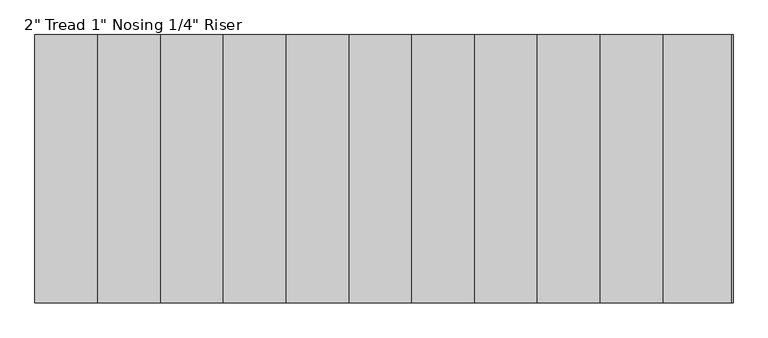
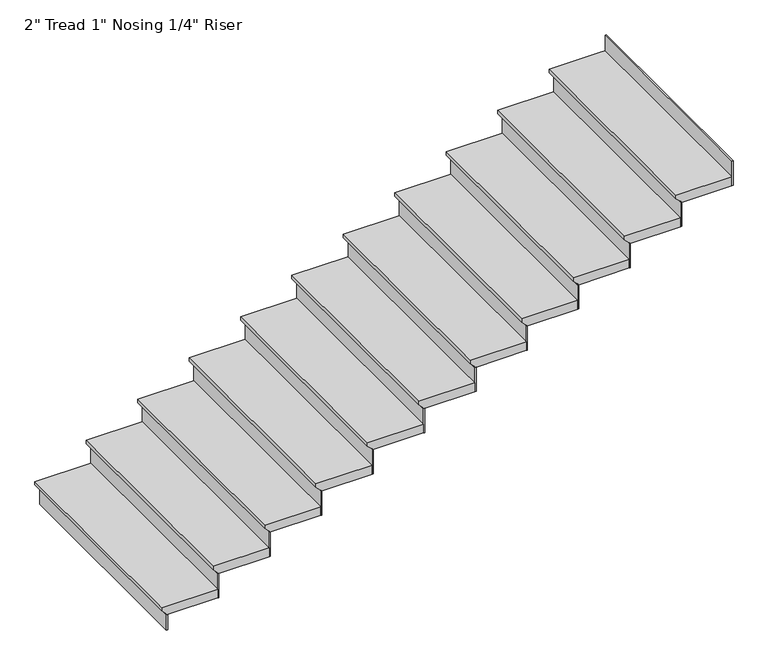
"""IFC4 building model written with IfcOpenShell, lengths in millimetres: stair flight geometry."""

from ifc_helpers import new_model, si_unit, origin, place, context, project, spatial, faceted_brep, source, transform, mapped, element, save


def stair_flight_1a668dfb(model_context):
    return source(origin(), model_context, "Body", "Brep", [
        faceted_brep([(-12936.8532683, 2168.0393562, 120.0978261), (-12936.8532683, 2168.0393562, 139.1478261), (-12936.8532683, 3361.8393562, 139.1478261), (-12936.8532683, 3361.8393562, 120.0978261), (-12911.4532683, 2168.0393562, 94.6978261), (-12911.4532683, 3361.8393562, 94.6978261), (-12632.0532683, 2168.0393562, 139.1478261), (-12632.0532683, 3361.8393562, 139.1478261), (-12911.4532683, 3361.8393562, 88.3478261), (-12632.0532683, 3361.8393562, 88.3478261), (-12632.0532683, 2168.0393562, 88.3478261), (-12911.4532683, 2168.0393562, 88.3478261)], [[[0, 1, 2, 3]], [[4, 0, 3, 5]], [[2, 1, 6, 7]], [[8, 9, 10, 11]], [[2, 7, 9, 8, 5, 3]], [[8, 11, 4, 5]], [[6, 1, 0, 4, 11, 10]], [[7, 6, 10, 9]]]),
        faceted_brep([(-12911.4532683, 2168.0393562, 88.3478261), (-12911.4532683, 2168.0393562, 0.0), (-12905.1032683, 2168.0393562, 0.0), (-12905.1032683, 2168.0393562, 88.3478261), (-12911.4532683, 3361.8393562, 88.3478261), (-12905.1032683, 3361.8393562, 88.3478261), (-12905.1032683, 3361.8393562, 0.0), (-12911.4532683, 3361.8393562, 0.0)], [[[0, 1, 2, 3]], [[4, 5, 6, 7]], [[1, 0, 4, 7]], [[2, 1, 7, 6]], [[3, 2, 6, 5]], [[0, 3, 5, 4]]]),
        faceted_brep([(-12632.0532683, 2168.0393562, 227.4956522), (-12632.0532683, 2168.0393562, 88.3478261), (-12625.7032683, 2168.0393562, 88.3478261), (-12625.7032683, 2168.0393562, 227.4956522), (-12632.0532683, 3361.8393562, 227.4956522), (-12625.7032683, 3361.8393562, 227.4956522), (-12625.7032683, 3361.8393562, 88.3478261), (-12632.0532683, 3361.8393562, 88.3478261)], [[[0, 1, 2, 3]], [[4, 5, 6, 7]], [[1, 0, 4, 7]], [[2, 1, 7, 6]], [[3, 2, 6, 5]], [[0, 3, 5, 4]]]),
        faceted_brep([(-12657.4532683, 3361.8393562, 278.2956522), (-12657.4532683, 2168.0393562, 278.2956522), (-12352.6532683, 2168.0393562, 278.2956522), (-12352.6532683, 3361.8393562, 278.2956522), (-12632.0532683, 3361.8393562, 227.4956522), (-12352.6532683, 3361.8393562, 227.4956522), (-12352.6532683, 2168.0393562, 227.4956522), (-12632.0532683, 2168.0393562, 227.4956522), (-12632.0532683, 3361.8393562, 233.8456522), (-12657.4532683, 3361.8393562, 259.2456522), (-12632.0532683, 2168.0393562, 233.8456522), (-12657.4532683, 2168.0393562, 259.2456522)], [[[0, 1, 2, 3]], [[4, 5, 6, 7]], [[0, 3, 5, 4, 8, 9]], [[4, 7, 10, 8]], [[2, 1, 11, 10, 7, 6]], [[3, 2, 6, 5]], [[11, 1, 0, 9]], [[10, 11, 9, 8]]]),
        faceted_brep([(-12352.6532683, 2168.0393562, 366.6434783), (-12352.6532683, 2168.0393562, 227.4956522), (-12346.3032683, 2168.0393562, 227.4956522), (-12346.3032683, 2168.0393562, 366.6434783), (-12352.6532683, 3361.8393562, 366.6434783), (-12346.3032683, 3361.8393562, 366.6434783), (-12346.3032683, 3361.8393562, 227.4956522), (-12352.6532683, 3361.8393562, 227.4956522)], [[[0, 1, 2, 3]], [[4, 5, 6, 7]], [[1, 0, 4, 7]], [[2, 1, 7, 6]], [[3, 2, 6, 5]], [[0, 3, 5, 4]]]),
        faceted_brep([(-12378.0532683, 3361.8393562, 417.4434783), (-12378.0532683, 2168.0393562, 417.4434783), (-12073.2532683, 2168.0393562, 417.4434783), (-12073.2532683, 3361.8393562, 417.4434783), (-12352.6532683, 3361.8393562, 366.6434783), (-12073.2532683, 3361.8393562, 366.6434783), (-12073.2532683, 2168.0393562, 366.6434783), (-12352.6532683, 2168.0393562, 366.6434783), (-12352.6532683, 3361.8393562, 372.9934783), (-12378.0532683, 3361.8393562, 398.3934783), (-12352.6532683, 2168.0393562, 372.9934783), (-12378.0532683, 2168.0393562, 398.3934783)], [[[0, 1, 2, 3]], [[4, 5, 6, 7]], [[0, 3, 5, 4, 8, 9]], [[4, 7, 10, 8]], [[2, 1, 11, 10, 7, 6]], [[3, 2, 6, 5]], [[11, 1, 0, 9]], [[10, 11, 9, 8]]]),
        faceted_brep([(-12073.2532683, 2168.0393562, 505.7913043), (-12073.2532683, 2168.0393562, 366.6434783), (-12066.9032683, 2168.0393562, 366.6434783), (-12066.9032683, 2168.0393562, 505.7913043), (-12073.2532683, 3361.8393562, 505.7913043), (-12066.9032683, 3361.8393562, 505.7913043), (-12066.9032683, 3361.8393562, 366.6434783), (-12073.2532683, 3361.8393562, 366.6434783)], [[[0, 1, 2, 3]], [[4, 5, 6, 7]], [[1, 0, 4, 7]], [[2, 1, 7, 6]], [[3, 2, 6, 5]], [[0, 3, 5, 4]]]),
        faceted_brep([(-12098.6532683, 3361.8393562, 556.5913043), (-12098.6532683, 2168.0393562, 556.5913043), (-11793.8532683, 2168.0393562, 556.5913043), (-11793.8532683, 3361.8393562, 556.5913043), (-12073.2532683, 3361.8393562, 505.7913043), (-11793.8532683, 3361.8393562, 505.7913043), (-11793.8532683, 2168.0393562, 505.7913043), (-12073.2532683, 2168.0393562, 505.7913043), (-12073.2532683, 3361.8393562, 512.1413043), (-12098.6532683, 3361.8393562, 537.5413043), (-12073.2532683, 2168.0393562, 512.1413043), (-12098.6532683, 2168.0393562, 537.5413043)], [[[0, 1, 2, 3]], [[4, 5, 6, 7]], [[0, 3, 5, 4, 8, 9]], [[4, 7, 10, 8]], [[2, 1, 11, 10, 7, 6]], [[3, 2, 6, 5]], [[11, 1, 0, 9]], [[10, 11, 9, 8]]]),
        faceted_brep([(-11793.8532683, 2168.0393562, 644.9391304), (-11793.8532683, 2168.0393562, 505.7913043), (-11787.5032683, 2168.0393562, 505.7913043), (-11787.5032683, 2168.0393562, 644.9391304), (-11793.8532683, 3361.8393562, 644.9391304), (-11787.5032683, 3361.8393562, 644.9391304), (-11787.5032683, 3361.8393562, 505.7913043), (-11793.8532683, 3361.8393562, 505.7913043)], [[[0, 1, 2, 3]], [[4, 5, 6, 7]], [[1, 0, 4, 7]], [[2, 1, 7, 6]], [[3, 2, 6, 5]], [[0, 3, 5, 4]]]),
        faceted_brep([(-11819.2532683, 3361.8393562, 695.7391304), (-11819.2532683, 2168.0393562, 695.7391304), (-11514.4532683, 2168.0393562, 695.7391304), (-11514.4532683, 3361.8393562, 695.7391304), (-11793.8532683, 3361.8393562, 644.9391304), (-11514.4532683, 3361.8393562, 644.9391304), (-11514.4532683, 2168.0393562, 644.9391304), (-11793.8532683, 2168.0393562, 644.9391304), (-11793.8532683, 3361.8393562, 651.2891304), (-11819.2532683, 3361.8393562, 676.6891304), (-11793.8532683, 2168.0393562, 651.2891304), (-11819.2532683, 2168.0393562, 676.6891304)], [[[0, 1, 2, 3]], [[4, 5, 6, 7]], [[0, 3, 5, 4, 8, 9]], [[4, 7, 10, 8]], [[2, 1, 11, 10, 7, 6]], [[3, 2, 6, 5]], [[11, 1, 0, 9]], [[10, 11, 9, 8]]]),
        faceted_brep([(-11514.4532683, 2168.0393562, 784.0869565), (-11514.4532683, 2168.0393562, 644.9391304), (-11508.1032683, 2168.0393562, 644.9391304), (-11508.1032683, 2168.0393562, 784.0869565), (-11514.4532683, 3361.8393562, 784.0869565), (-11508.1032683, 3361.8393562, 784.0869565), (-11508.1032683, 3361.8393562, 644.9391304), (-11514.4532683, 3361.8393562, 644.9391304)], [[[0, 1, 2, 3]], [[4, 5, 6, 7]], [[1, 0, 4, 7]], [[2, 1, 7, 6]], [[3, 2, 6, 5]], [[0, 3, 5, 4]]]),
        faceted_brep([(-11539.8532683, 3361.8393562, 834.8869565), (-11539.8532683, 2168.0393562, 834.8869565), (-11235.0532683, 2168.0393562, 834.8869565), (-11235.0532683, 3361.8393562, 834.8869565), (-11514.4532683, 3361.8393562, 784.0869565), (-11235.0532683, 3361.8393562, 784.0869565), (-11235.0532683, 2168.0393562, 784.0869565), (-11514.4532683, 2168.0393562, 784.0869565), (-11514.4532683, 3361.8393562, 790.4369565), (-11539.8532683, 3361.8393562, 815.8369565), (-11514.4532683, 2168.0393562, 790.4369565), (-11539.8532683, 2168.0393562, 815.8369565)], [[[0, 1, 2, 3]], [[4, 5, 6, 7]], [[0, 3, 5, 4, 8, 9]], [[4, 7, 10, 8]], [[2, 1, 11, 10, 7, 6]], [[3, 2, 6, 5]], [[11, 1, 0, 9]], [[10, 11, 9, 8]]]),
        faceted_brep([(-11235.0532683, 2168.0393562, 923.2347826), (-11235.0532683, 2168.0393562, 784.0869565), (-11228.7032683, 2168.0393562, 784.0869565), (-11228.7032683, 2168.0393562, 923.2347826), (-11235.0532683, 3361.8393562, 923.2347826), (-11228.7032683, 3361.8393562, 923.2347826), (-11228.7032683, 3361.8393562, 784.0869565), (-11235.0532683, 3361.8393562, 784.0869565)], [[[0, 1, 2, 3]], [[4, 5, 6, 7]], [[1, 0, 4, 7]], [[2, 1, 7, 6]], [[3, 2, 6, 5]], [[0, 3, 5, 4]]]),
        faceted_brep([(-11260.4532683, 3361.8393562, 974.0347826), (-11260.4532683, 2168.0393562, 974.0347826), (-10955.6532683, 2168.0393562, 974.0347826), (-10955.6532683, 3361.8393562, 974.0347826), (-11235.0532683, 3361.8393562, 923.2347826), (-10955.6532683, 3361.8393562, 923.2347826), (-10955.6532683, 2168.0393562, 923.2347826), (-11235.0532683, 2168.0393562, 923.2347826), (-11235.0532683, 3361.8393562, 929.5847826), (-11260.4532683, 3361.8393562, 954.9847826), (-11235.0532683, 2168.0393562, 929.5847826), (-11260.4532683, 2168.0393562, 954.9847826)], [[[0, 1, 2, 3]], [[4, 5, 6, 7]], [[0, 3, 5, 4, 8, 9]], [[4, 7, 10, 8]], [[2, 1, 11, 10, 7, 6]], [[3, 2, 6, 5]], [[11, 1, 0, 9]], [[10, 11, 9, 8]]]),
        faceted_brep([(-10955.6532683, 2168.0393562, 1062.3826087), (-10955.6532683, 2168.0393562, 923.2347826), (-10949.3032683, 2168.0393562, 923.2347826), (-10949.3032683, 2168.0393562, 1062.3826087), (-10955.6532683, 3361.8393562, 1062.3826087), (-10949.3032683, 3361.8393562, 1062.3826087), (-10949.3032683, 3361.8393562, 923.2347826), (-10955.6532683, 3361.8393562, 923.2347826)], [[[0, 1, 2, 3]], [[4, 5, 6, 7]], [[1, 0, 4, 7]], [[2, 1, 7, 6]], [[3, 2, 6, 5]], [[0, 3, 5, 4]]]),
        faceted_brep([(-10981.0532683, 3361.8393562, 1113.1826087), (-10981.0532683, 2168.0393562, 1113.1826087), (-10676.2532683, 2168.0393562, 1113.1826087), (-10676.2532683, 3361.8393562, 1113.1826087), (-10955.6532683, 3361.8393562, 1062.3826087), (-10676.2532683, 3361.8393562, 1062.3826087), (-10676.2532683, 2168.0393562, 1062.3826087), (-10955.6532683, 2168.0393562, 1062.3826087), (-10955.6532683, 3361.8393562, 1068.7326087), (-10981.0532683, 3361.8393562, 1094.1326087), (-10955.6532683, 2168.0393562, 1068.7326087), (-10981.0532683, 2168.0393562, 1094.1326087)], [[[0, 1, 2, 3]], [[4, 5, 6, 7]], [[0, 3, 5, 4, 8, 9]], [[4, 7, 10, 8]], [[2, 1, 11, 10, 7, 6]], [[3, 2, 6, 5]], [[11, 1, 0, 9]], [[10, 11, 9, 8]]]),
        faceted_brep([(-10676.2532683, 2168.0393562, 1201.5304348), (-10676.2532683, 2168.0393562, 1062.3826087), (-10669.9032683, 2168.0393562, 1062.3826087), (-10669.9032683, 2168.0393562, 1201.5304348), (-10676.2532683, 3361.8393562, 1201.5304348), (-10669.9032683, 3361.8393562, 1201.5304348), (-10669.9032683, 3361.8393562, 1062.3826087), (-10676.2532683, 3361.8393562, 1062.3826087)], [[[0, 1, 2, 3]], [[4, 5, 6, 7]], [[1, 0, 4, 7]], [[2, 1, 7, 6]], [[3, 2, 6, 5]], [[0, 3, 5, 4]]]),
        faceted_brep([(-10701.6532683, 3361.8393562, 1252.3304348), (-10701.6532683, 2168.0393562, 1252.3304348), (-10396.8532683, 2168.0393562, 1252.3304348), (-10396.8532683, 3361.8393562, 1252.3304348), (-10676.2532683, 3361.8393562, 1201.5304348), (-10396.8532683, 3361.8393562, 1201.5304348), (-10396.8532683, 2168.0393562, 1201.5304348), (-10676.2532683, 2168.0393562, 1201.5304348), (-10676.2532683, 3361.8393562, 1207.8804348), (-10701.6532683, 3361.8393562, 1233.2804348), (-10676.2532683, 2168.0393562, 1207.8804348), (-10701.6532683, 2168.0393562, 1233.2804348)], [[[0, 1, 2, 3]], [[4, 5, 6, 7]], [[0, 3, 5, 4, 8, 9]], [[4, 7, 10, 8]], [[2, 1, 11, 10, 7, 6]], [[3, 2, 6, 5]], [[11, 1, 0, 9]], [[10, 11, 9, 8]]]),
        faceted_brep([(-10396.8532683, 2168.0393562, 1340.6782609), (-10396.8532683, 2168.0393562, 1201.5304348), (-10390.5032683, 2168.0393562, 1201.5304348), (-10390.5032683, 2168.0393562, 1340.6782609), (-10396.8532683, 3361.8393562, 1340.6782609), (-10390.5032683, 3361.8393562, 1340.6782609), (-10390.5032683, 3361.8393562, 1201.5304348), (-10396.8532683, 3361.8393562, 1201.5304348)], [[[0, 1, 2, 3]], [[4, 5, 6, 7]], [[1, 0, 4, 7]], [[2, 1, 7, 6]], [[3, 2, 6, 5]], [[0, 3, 5, 4]]]),
        faceted_brep([(-10422.2532683, 3361.8393562, 1391.4782609), (-10422.2532683, 2168.0393562, 1391.4782609), (-10117.4532683, 2168.0393562, 1391.4782609), (-10117.4532683, 3361.8393562, 1391.4782609), (-10396.8532683, 3361.8393562, 1340.6782609), (-10117.4532683, 3361.8393562, 1340.6782609), (-10117.4532683, 2168.0393562, 1340.6782609), (-10396.8532683, 2168.0393562, 1340.6782609), (-10396.8532683, 3361.8393562, 1347.0282609), (-10422.2532683, 3361.8393562, 1372.4282609), (-10396.8532683, 2168.0393562, 1347.0282609), (-10422.2532683, 2168.0393562, 1372.4282609)], [[[0, 1, 2, 3]], [[4, 5, 6, 7]], [[0, 3, 5, 4, 8, 9]], [[4, 7, 10, 8]], [[2, 1, 11, 10, 7, 6]], [[3, 2, 6, 5]], [[11, 1, 0, 9]], [[10, 11, 9, 8]]]),
        faceted_brep([(-9838.0532683, 2168.0393562, 1618.973913), (-9838.0532683, 2168.0393562, 1479.826087), (-9831.7032683, 2168.0393562, 1479.826087), (-9831.7032683, 2168.0393562, 1618.973913), (-9838.0532683, 3361.8393562, 1618.973913), (-9831.7032683, 3361.8393562, 1618.973913), (-9831.7032683, 3361.8393562, 1479.826087), (-9838.0532683, 3361.8393562, 1479.826087)], [[[0, 1, 2, 3]], [[4, 5, 6, 7]], [[1, 0, 4, 7]], [[2, 1, 7, 6]], [[3, 2, 6, 5]], [[0, 3, 5, 4]]]),
        faceted_brep([(-10117.4532683, 2168.0393562, 1479.826087), (-10117.4532683, 2168.0393562, 1340.6782609), (-10111.1032683, 2168.0393562, 1340.6782609), (-10111.1032683, 2168.0393562, 1479.826087), (-10117.4532683, 3361.8393562, 1479.826087), (-10111.1032683, 3361.8393562, 1479.826087), (-10111.1032683, 3361.8393562, 1340.6782609), (-10117.4532683, 3361.8393562, 1340.6782609)], [[[0, 1, 2, 3]], [[4, 5, 6, 7]], [[1, 0, 4, 7]], [[2, 1, 7, 6]], [[3, 2, 6, 5]], [[0, 3, 5, 4]]]),
        faceted_brep([(-9838.0532683, 3361.8393562, 1530.626087), (-9863.4532683, 3361.8393562, 1530.626087), (-10142.8532683, 3361.8393562, 1530.626087), (-10142.8532683, 2168.0393562, 1530.626087), (-9838.0532683, 2168.0393562, 1530.626087), (-9863.4532683, 3361.8393562, 1479.826087), (-9838.0532683, 3361.8393562, 1479.826087), (-9838.0532683, 2168.0393562, 1479.826087), (-10117.4532683, 2168.0393562, 1479.826087), (-10117.4532683, 3361.8393562, 1479.826087), (-10117.4532683, 3361.8393562, 1486.176087), (-10142.8532683, 3361.8393562, 1511.576087), (-10117.4532683, 2168.0393562, 1486.176087), (-10142.8532683, 2168.0393562, 1511.576087)], [[[0, 1, 2, 3, 4]], [[5, 6, 7, 8, 9]], [[1, 0, 6, 5]], [[2, 1, 5, 9, 10, 11]], [[9, 8, 12, 10]], [[4, 3, 13, 12, 8, 7]], [[0, 4, 7, 6]], [[13, 3, 2, 11]], [[12, 13, 11, 10]]]),
    ])


if __name__ == "__main__":
    model = new_model("IFC4")
    model_context = context("Model", 3, world=origin())
    ifc_project = project(units=[si_unit("LENGTHUNIT", "METRE", prefix="MILLI")], contexts=[model_context])
    site = spatial("IfcSite", under=ifc_project)
    building = spatial("IfcBuilding", under=site)
    placement = place(None, origin())
    stair_flight_shape = stair_flight_1a668dfb(model_context)
    element("IfcStairFlight", 1, ObjectType="2\" Tread 1\" Nosing 1/4\" Riser", at=placement, inside=building, context=model_context, shape_type="MappedRepresentation", body=[
        mapped(stair_flight_shape, transform((0.0, 0.0, 0.0), x_axis=(1.0, 0.0, 0.0), y_axis=(0.0, 1.0, 0.0), z_axis=(0.0, 0.0, 1.0))),
    ])
    save(model, "model.ifc")
